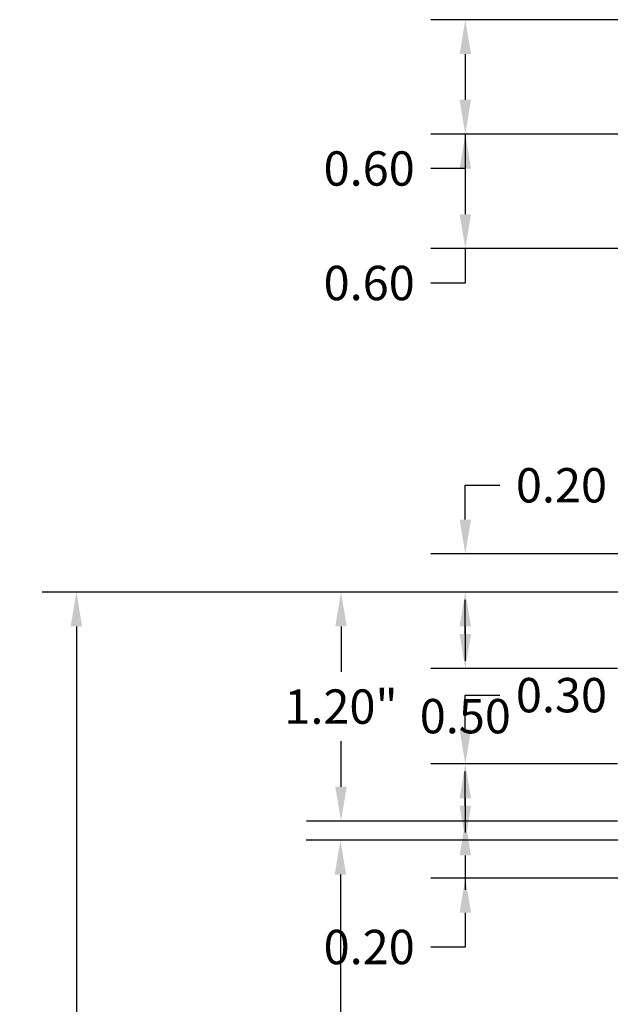
# Model space of a CAD drawing. Units: metres. Extents: x -1.9 to 13.1, y 0.9 to 14.8.
# Tile 4 of 7: x -1.9 to 1.2, y 8.4 to 13.6. Entities that reach past the tile are written whole.
import ezdxf

# ---------------------------------------------------------------- set-up
doc = ezdxf.new("R2010")
doc.units = ezdxf.units.M
doc.header["$MEASUREMENT"] = 0
doc.layers.add('A-ANNO-DIMS', color=2, linetype='Continuous', lineweight=13)
doc.styles.get("Standard").update_dxf_attribs({"font": 'arial.ttf'})
doc.dimstyles.get("Standard").update_dxf_attribs({"dimtxt": 0.18, "dimasz": 0.18, "dimexe": 0.18, "dimexo": 0.0625, "dimgap": 0.09, "dimtad": 0, "dimtih": 1, "dimtoh": 1, "dimzin": 0, "dimdsep": 46, "dimlunit": 3, "dimtxsty": 'Standard', "dimcen": 0.09, "dimadec": 0, "dimazin": 0, "dimtfac": 1, "dimtofl": 0, "dimtmove": 0, "dimatfit": 3, "dimfxl": 1, "dimtolj": 1, "dimtzin": 0, "dimarcsym": 0})

# ---------------------------------------------------------------- blocks, each defined once
blk = doc.blocks.new('*D20')
at = {"layer": 'A-ANNO-DIMS', "color": 0, "lineweight": -2, "transparency": 16777216}
for p, q in [((1.1413, 10.5964), (-1.7723, 10.5964)), ((-1.5923, 10.4164), (-1.5923, 6.8283)), ((-1.5923, 2.8764), (-1.5923, 6.4645)), ((1.1413, 2.6964), (-1.7723, 2.6964))]:
    blk.add_line(p, q, dxfattribs=at)
at = {"layer": 'A-ANNO-DIMS', "color": 0, "transparency": 16777216}
for points in [[(-1.6223, 10.4164), (-1.5623, 10.4164), (-1.5923, 10.5964)], [(-1.6223, 2.8764), (-1.5623, 2.8764), (-1.5923, 2.6964)]]:
    blk.add_solid(points, dxfattribs=at)
at = {"layer": 'Defpoints', "color": 0, "transparency": 16777216}
for p in [(1.2038, 10.5964), (-1.5923, 2.6964), (1.2038, 2.6964)]:
    blk.add_point(p, dxfattribs=at)
at = {"layer": 'A-ANNO-DIMS', "color": 0, "transparency": 16777216, "insert": (-1.5923, 6.6464), "char_height": 0.18, "attachment_point": 5}
blk.add_mtext('\\A1;7.90"', dxfattribs=at)
blk = doc.blocks.new('*D21')
at = {"layer": 'A-ANNO-DIMS', "color": 0, "lineweight": -2, "transparency": 16777216}
for p, q in [((1.1413, 10.5964), (-0.3866, 10.5964)), ((-0.2066, 10.4164), (-0.2066, 10.1783)), ((-0.2066, 9.5764), (-0.2066, 9.8145)), ((1.1413, 9.3964), (-0.3866, 9.3964))]:
    blk.add_line(p, q, dxfattribs=at)
at = {"layer": 'A-ANNO-DIMS', "color": 0, "transparency": 16777216}
for points in [[(-0.2366, 10.4164), (-0.1766, 10.4164), (-0.2066, 10.5964)], [(-0.2366, 9.5764), (-0.1766, 9.5764), (-0.2066, 9.3964)]]:
    blk.add_solid(points, dxfattribs=at)
at = {"layer": 'Defpoints', "color": 0, "transparency": 16777216}
for p in [(1.2038, 10.5964), (-0.2066, 9.3964), (1.2038, 9.3964)]:
    blk.add_point(p, dxfattribs=at)
at = {"layer": 'A-ANNO-DIMS', "color": 0, "transparency": 16777216, "insert": (-0.2066, 9.9964), "char_height": 0.18, "attachment_point": 5}
blk.add_mtext('\\A1;1.20"', dxfattribs=at)
blk = doc.blocks.new('*D22')
at = {"layer": 'A-ANNO-DIMS', "color": 0, "lineweight": -2, "transparency": 16777216}
for p, q in [((1.1413, 9.2964), (-0.3896, 9.2964)), ((-0.2096, 9.1164), (-0.2096, 7.7756)), ((-0.2096, 6.0709), (-0.2096, 7.4117)), ((1.1413, 5.8909), (-0.3896, 5.8909))]:
    blk.add_line(p, q, dxfattribs=at)
at = {"layer": 'A-ANNO-DIMS', "color": 0, "transparency": 16777216}
for points in [[(-0.2396, 9.1164), (-0.1796, 9.1164), (-0.2096, 9.2964)], [(-0.2396, 6.0709), (-0.1796, 6.0709), (-0.2096, 5.8909)]]:
    blk.add_solid(points, dxfattribs=at)
at = {"layer": 'Defpoints', "color": 0, "transparency": 16777216}
for p in [(1.2038, 9.2964), (-0.2096, 5.8909), (1.2038, 5.8909)]:
    blk.add_point(p, dxfattribs=at)
at = {"layer": 'A-ANNO-DIMS', "color": 0, "transparency": 16777216, "insert": (-0.2096, 7.5936), "char_height": 0.18, "attachment_point": 5}
blk.add_mtext('\\A1;3.41"', dxfattribs=at)
blk = doc.blocks.new('*D53')
at = {"layer": 'A-ANNO-DIMS', "color": 0, "lineweight": -2, "transparency": 16777216}
for p, q in [((0.4443, 9.8764), (0.4443, 10.0564)), ((0.4443, 10.0564), (0.6243, 10.0564)), ((1.2413, 9.6964), (0.2643, 9.6964)), ((1.2413, 9.3964), (0.2643, 9.3964)), ((0.4443, 9.2164), (0.4443, 9.0364))]:
    blk.add_line(p, q, dxfattribs=at)
at = {"layer": 'A-ANNO-DIMS', "color": 0, "transparency": 16777216}
for points in [[(0.4143, 9.8764), (0.4743, 9.8764), (0.4443, 9.6964)], [(0.4143, 9.2164), (0.4743, 9.2164), (0.4443, 9.3964)]]:
    blk.add_solid(points, dxfattribs=at)
at = {"layer": 'Defpoints', "color": 0, "transparency": 16777216}
for p in [(0.4443, 9.6964), (1.3038, 9.6964), (1.3038, 9.3964)]:
    blk.add_point(p, dxfattribs=at)
at = {"layer": 'A-ANNO-DIMS', "color": 0, "transparency": 16777216, "insert": (0.9478, 10.0564), "char_height": 0.18, "attachment_point": 5}
blk.add_mtext('\\A1;0.30', dxfattribs=at)
blk = doc.blocks.new('*D54')
at = {"layer": 'A-ANNO-DIMS', "color": 0, "lineweight": -2, "transparency": 16777216}
for p, q in [((0.444347, 10.376378), (0.444347, 10.556378)), ((1.241347, 10.196378), (0.264347, 10.196378)), ((1.241347, 9.696378), (0.264347, 9.696378)), ((0.444347, 9.516378), (0.444347, 9.336378))]:
    blk.add_line(p, q, dxfattribs=at)
at = {"layer": 'A-ANNO-DIMS', "color": 0, "transparency": 16777216}
for points in [[(0.414347, 10.376378), (0.474347, 10.376378), (0.444347, 10.196378)], [(0.414347, 9.516378), (0.474347, 9.516378), (0.444347, 9.696378)]]:
    blk.add_solid(points, dxfattribs=at)
at = {"layer": 'Defpoints', "color": 0, "transparency": 16777216}
for p in [(0.444347, 10.196378), (1.303847, 10.196378), (1.303847, 9.696378)]:
    blk.add_point(p, dxfattribs=at)
at = {"layer": 'A-ANNO-DIMS', "color": 0, "transparency": 16777216, "insert": (0.444347, 9.946378), "char_height": 0.18, "attachment_point": 5}
blk.add_mtext('\\A1;0.50', dxfattribs=at)
blk = doc.blocks.new('*D62')
at = {"layer": 'A-ANNO-DIMS', "color": 0, "lineweight": -2, "transparency": 16777216}
for p, q in [((0.4443, 10.9764), (0.4443, 11.1564)), ((0.4443, 11.1564), (0.6243, 11.1564)), ((2.8413, 10.7964), (0.2643, 10.7964)), ((2.8413, 10.5964), (0.2643, 10.5964)), ((0.4443, 10.4164), (0.4443, 10.2364))]:
    blk.add_line(p, q, dxfattribs=at)
at = {"layer": 'A-ANNO-DIMS', "color": 0, "transparency": 16777216}
for points in [[(0.4143, 10.9764), (0.4743, 10.9764), (0.4443, 10.7964)], [(0.4143, 10.4164), (0.4743, 10.4164), (0.4443, 10.5964)]]:
    blk.add_solid(points, dxfattribs=at)
at = {"layer": 'Defpoints', "color": 0, "transparency": 16777216}
for p in [(0.4443, 10.7964), (2.9038, 10.7964), (2.9038, 10.5964)]:
    blk.add_point(p, dxfattribs=at)
at = {"layer": 'A-ANNO-DIMS', "color": 0, "transparency": 16777216, "insert": (0.9478, 11.1564), "char_height": 0.18, "attachment_point": 5}
blk.add_mtext('\\A1;0.20', dxfattribs=at)
blk = doc.blocks.new('*D63')
at = {"layer": 'A-ANNO-DIMS', "color": 0, "lineweight": -2, "transparency": 16777216}
for p, q in [((0.4443, 9.4764), (0.4443, 9.6564)), ((3.7413, 9.2964), (0.2643, 9.2964)), ((3.7413, 9.0964), (0.2643, 9.0964)), ((0.4443, 8.9164), (0.4443, 8.7364)), ((0.4443, 8.7364), (0.2643, 8.7364))]:
    blk.add_line(p, q, dxfattribs=at)
at = {"layer": 'A-ANNO-DIMS', "color": 0, "transparency": 16777216}
for points in [[(0.4143, 9.4764), (0.4743, 9.4764), (0.4443, 9.2964)], [(0.4143, 8.9164), (0.4743, 8.9164), (0.4443, 9.0964)]]:
    blk.add_solid(points, dxfattribs=at)
at = {"layer": 'Defpoints', "color": 0, "transparency": 16777216}
for p in [(3.8038, 9.2964), (0.4443, 9.0964), (3.8038, 9.0964)]:
    blk.add_point(p, dxfattribs=at)
at = {"layer": 'A-ANNO-DIMS', "color": 0, "transparency": 16777216, "insert": (-0.0591, 8.7364), "char_height": 0.18, "attachment_point": 5}
blk.add_mtext('\\A1;0.20', dxfattribs=at)
blk = doc.blocks.new('*D71')
at = {"layer": 'A-ANNO-DIMS', "color": 0, "lineweight": -2, "transparency": 16777216}
for p, q in [((2.9413, 13.5964), (0.2643, 13.5964)), ((0.4443, 13.4164), (0.4443, 13.1764)), ((2.9413, 12.9964), (0.2643, 12.9964)), ((0.4443, 12.9964), (0.4443, 12.8164)), ((0.4443, 12.8164), (0.2643, 12.8164))]:
    blk.add_line(p, q, dxfattribs=at)
at = {"layer": 'A-ANNO-DIMS', "color": 0, "transparency": 16777216}
for points in [[(0.4143, 13.4164), (0.4743, 13.4164), (0.4443, 13.5964)], [(0.4143, 13.1764), (0.4743, 13.1764), (0.4443, 12.9964)]]:
    blk.add_solid(points, dxfattribs=at)
at = {"layer": 'Defpoints', "color": 0, "transparency": 16777216}
for p in [(3.0038, 13.5964), (0.4443, 12.9964), (3.0038, 12.9964)]:
    blk.add_point(p, dxfattribs=at)
at = {"layer": 'A-ANNO-DIMS', "color": 0, "transparency": 16777216, "insert": (-0.0591, 12.8164), "char_height": 0.18, "attachment_point": 5}
blk.add_mtext('\\A1;0.60', dxfattribs=at)
blk = doc.blocks.new('*D72')
at = {"layer": 'A-ANNO-DIMS', "color": 0, "lineweight": -2, "transparency": 16777216}
for p, q in [((2.9413, 12.9964), (0.2643, 12.9964)), ((0.4443, 12.8164), (0.4443, 12.5764)), ((2.9413, 12.3964), (0.2643, 12.3964)), ((0.4443, 12.3964), (0.4443, 12.2164)), ((0.4443, 12.2164), (0.2643, 12.2164))]:
    blk.add_line(p, q, dxfattribs=at)
at = {"layer": 'A-ANNO-DIMS', "color": 0, "transparency": 16777216}
for points in [[(0.4143, 12.8164), (0.4743, 12.8164), (0.4443, 12.9964)], [(0.4143, 12.5764), (0.4743, 12.5764), (0.4443, 12.3964)]]:
    blk.add_solid(points, dxfattribs=at)
at = {"layer": 'Defpoints', "color": 0, "transparency": 16777216}
for p in [(3.0038, 12.9964), (0.4443, 12.3964), (3.0038, 12.3964)]:
    blk.add_point(p, dxfattribs=at)
at = {"layer": 'A-ANNO-DIMS', "color": 0, "transparency": 16777216, "insert": (-0.0591, 12.2164), "char_height": 0.18, "attachment_point": 5}
blk.add_mtext('\\A1;0.60', dxfattribs=at)

msp = doc.modelspace()

# ---------------------------------------------------------------- dimensions: what is measured, and where the dimension line sits
at = {"layer": 'A-ANNO-DIMS'}
for base, p1, p2, override, picture, middle in [((0.4443, 12.9964), (3.0038, 13.5964), (3.0038, 12.9964), {"dimdec": 2, "dimlfac": 1, "dimrnd": 0, "dimzin": 0, "dimdsep": 46, "dimlunit": 2}, '*D71', (-0.0591, 12.8164)), ((0.4443, 12.3964), (3.0038, 12.9964), (3.0038, 12.3964), {"dimdec": 2, "dimlfac": 1, "dimrnd": 0, "dimzin": 0, "dimdsep": 46, "dimlunit": 2}, '*D72', (-0.0591, 12.2164)), ((0.4443, 10.7964), (2.9038, 10.5964), (2.9038, 10.7964), {"dimdec": 2, "dimlfac": 1, "dimrnd": 0, "dimzin": 0, "dimdsep": 46, "dimlunit": 2}, '*D62', (0.9478, 11.1564)), ((-1.5923, 2.6964), (1.2038, 10.5964), (1.2038, 2.6964), {"dimclrd": 0, "dimclre": 0, "dimclrt": 0}, '*D20', (-1.5923, 6.6464)), ((-0.2066, 9.3964), (1.2038, 10.5964), (1.2038, 9.3964), {"dimclrd": 0, "dimclre": 0, "dimclrt": 0}, '*D21', (-0.2066, 9.9964)), ((0.4443, 10.1964), (1.3038, 9.6964), (1.3038, 10.1964), {"dimdec": 2, "dimlfac": 1, "dimrnd": 0, "dimzin": 0, "dimdsep": 46, "dimlunit": 2}, '*D54', (0.4443, 9.9464)), ((0.4443, 9.6964), (1.3038, 9.3964), (1.3038, 9.6964), {"dimdec": 2, "dimlfac": 1, "dimrnd": 0, "dimzin": 0, "dimdsep": 46, "dimlunit": 2}, '*D53', (0.9478, 10.0564)), ((0.4443, 9.0964), (3.8038, 9.2964), (3.8038, 9.0964), {"dimdec": 2, "dimlfac": 1, "dimrnd": 0, "dimzin": 0, "dimdsep": 46, "dimlunit": 2}, '*D63', (-0.0591, 8.7364)), ((-0.2096, 5.8909), (1.2038, 9.2964), (1.2038, 5.8909), {"dimclrd": 0, "dimclre": 0, "dimclrt": 0}, '*D22', (-0.2096, 7.5936))]:
    dim = msp.add_linear_dim(base=base, p1=p1, p2=p2, angle=90, dimstyle='Standard', override=override, dxfattribs=at)
    dim.commit()
    dim.dimension.update_dxf_attribs({"geometry": picture, "text_midpoint": middle})

doc.saveas('drawing.dxf')
